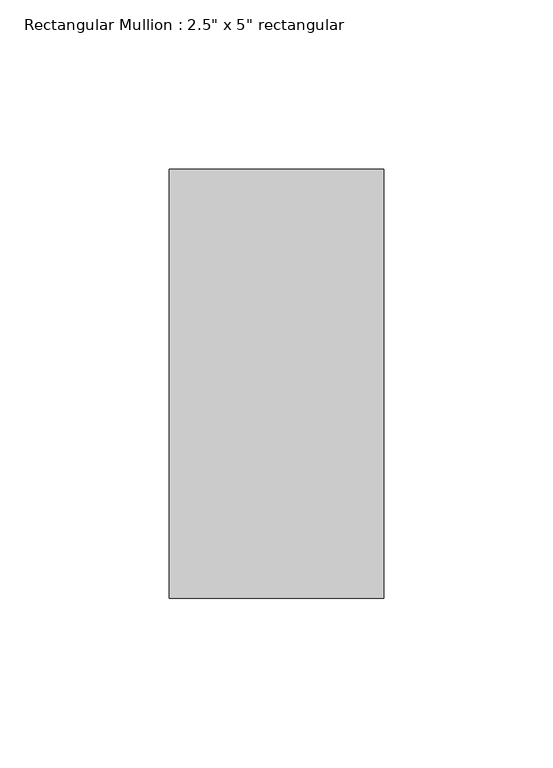
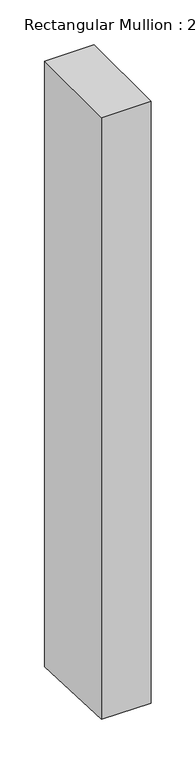
"""IFC4 building model written with IfcOpenShell, lengths in millimetres: member geometry."""

from ifc_helpers import new_model, si_unit, frame, origin, place, context, project, spatial, polyline, outline, extrude, source, transform, mapped, element, save


def member_868818ab(model_context):
    return source(origin(), model_context, "Body", "SweptSolid", [
        extrude(outline(polyline([(-63.5, 0.0), (63.5, 0.0), (63.5, -823.7980727), (-63.5, -818.6350785), (-63.5, 0.0)])), frame((-63.5, 0.0, 0.0), z_axis=(1.0, 0.0, 0.0), x_axis=(0.0, 1.0, 0.0)), (0.0, 0.0, 1.0), 63.5),
    ])


if __name__ == "__main__":
    model = new_model("IFC4")
    model_context = context("Model", 3, world=origin())
    ifc_project = project(units=[si_unit("LENGTHUNIT", "METRE", prefix="MILLI")], contexts=[model_context])
    site = spatial("IfcSite", under=ifc_project)
    building = spatial("IfcBuilding", under=site)
    placement = place(None, origin())
    member_shape = member_868818ab(model_context)
    element("IfcMember", 1, ObjectType="Rectangular Mullion : 2.5\" x 5\" rectangular", at=placement, inside=building, context=model_context, shape_type="MappedRepresentation", body=[
        mapped(member_shape, transform((0.0, 0.0, 0.0), x_axis=(1.0, 0.0, 0.0), y_axis=(0.0, 1.0, 0.0), z_axis=(0.0, 0.0, 1.0))),
    ])
    save(model, "model.ifc")

# Revit data of these elements
# Type "Rectangular Mullion : 2.5\" x 5\" rectangular"
#   built-in parameter 1007304 = 0.416667 (stored number, unit not read)
#   built-in parameter 1007301 = 0.104167 (stored number, unit not read)
#   built-in parameter 1007300 = 0.104167 (stored number, unit not read)
# Element 1 (IfcMember, "Rectangular Mullion : 2.5\" x 5\" rectangular")
#   Materials on its faces: "Aluminum"
# Materials
#   "Aluminum": class "Metal", colour RGB 247 247 247, transparency 0, Description = "Aluminum 6061", Cost = 0
